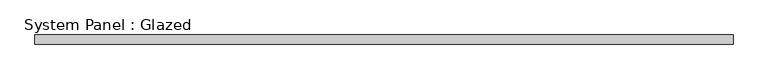
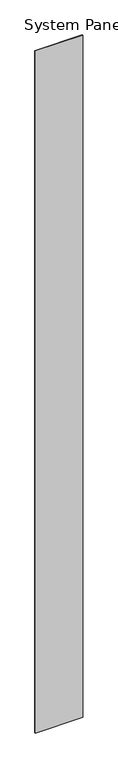
"""IFC4 building model written with IfcOpenShell, lengths in millimetres: plate geometry, System Panel : Glazed."""

from ifc_helpers import new_model, si_unit, origin, origin_with_axes, place, context, project, spatial, polyline, outline, extrude, source, transform, mapped, element, save


def system_panel_glazed_978fe6fd(model_context):
    return source(origin(), model_context, "Body", "SweptSolid", [
        extrude(outline(polyline([(958.85, 19.05), (-958.85, 19.05), (-958.85, 44.45), (958.85, 44.45), (958.85, 19.05)])), origin_with_axes(), (0.0, 0.0, 1.0), 29133.8),
    ])


if __name__ == "__main__":
    model = new_model("IFC4")
    model_context = context("Model", 3, world=origin())
    ifc_project = project(units=[si_unit("LENGTHUNIT", "METRE", prefix="MILLI")], contexts=[model_context])
    site = spatial("IfcSite", under=ifc_project)
    building = spatial("IfcBuilding", under=site)
    placement = place(None, origin())
    system_panel_glazed_shape = system_panel_glazed_978fe6fd(model_context)
    element("IfcPlate", 1, ObjectType="System Panel : Glazed", at=placement, inside=building, context=model_context, shape_type="MappedRepresentation", body=[
        mapped(system_panel_glazed_shape, transform((0.0, 0.0, 0.0), x_axis=(1.0, 0.0, 0.0), y_axis=(0.0, 1.0, 0.0), z_axis=(0.0, 0.0, 1.0))),
    ])
    save(model, "model.ifc")

# Revit data of these elements
# Type "System Panel : Glazed"
#   Construction Type Id = "GSP4R"
#   Analytic Construction = "1/8 in Pilkington single glazing"
#   Visual Light Transmittance = 0.9
#   Solar Heat Gain Coefficient = 0.86
#   Heat Transfer Coefficient (U) = 1.18115 BTU/(h·ft²·°F)
# Element 1 (IfcPlate, "System Panel : Glazed")
#   Materials on its faces: "Glass"
# Materials
#   "Glass": class "Glass", colour RGB 0 128 192, transparency 0.75, Description = "Soda Lime Glass", Cost = 0
